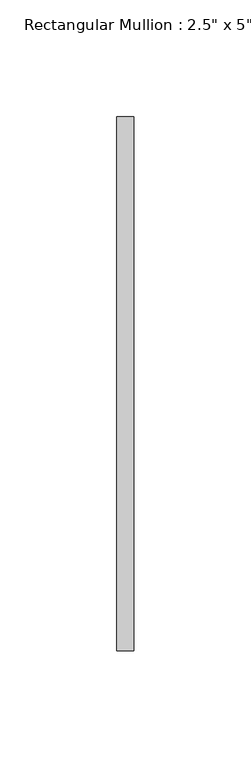
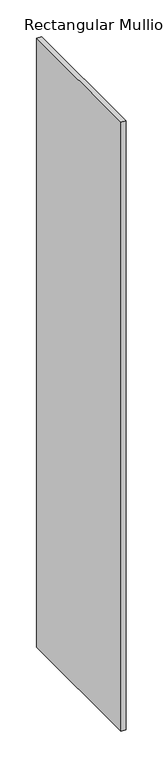
"""IFC4 building model written with IfcOpenShell, lengths in millimetres: member geometry."""

from ifc_helpers import new_model, si_unit, frame, origin, place, context, project, spatial, polyline, outline, extrude, source, transform, mapped, element, save


def member_9004b0e6(model_context):
    return source(origin(), model_context, "Body", "SweptSolid", [
        extrude(outline(polyline([(0.0, 114.3), (0.0, -114.3), (-7.239, -114.3), (-7.239, 114.3), (0.0, 114.3)])), frame((0.0, 0.0, -1005.1415), z_axis=(0.0, 0.0, 1.0), x_axis=(1.0, 0.0, 0.0)), (0.0, 0.0, 1.0), 1005.1415),
    ])


if __name__ == "__main__":
    model = new_model("IFC4")
    model_context = context("Model", 3, world=origin())
    ifc_project = project(units=[si_unit("LENGTHUNIT", "METRE", prefix="MILLI")], contexts=[model_context])
    site = spatial("IfcSite", under=ifc_project)
    building = spatial("IfcBuilding", under=site)
    placement = place(None, origin())
    member_shape = member_9004b0e6(model_context)
    element("IfcMember", 1, ObjectType="Rectangular Mullion : 2.5\" x 5\" rectangular", at=placement, inside=building, context=model_context, shape_type="MappedRepresentation", body=[
        mapped(member_shape, transform((0.0, 0.0, 0.0), x_axis=(1.0, 0.0, 0.0), y_axis=(0.0, 1.0, 0.0), z_axis=(0.0, 0.0, 1.0))),
    ])
    save(model, "model.ifc")

# Revit data of these elements
# Type "Rectangular Mullion : 2.5\" x 5\" rectangular"
#   built-in parameter 1007304 = 0.75 (stored number, unit not read)
#   built-in parameter 1007301 = 0.011875 (stored number, unit not read)
#   built-in parameter 1007300 = 0.011875 (stored number, unit not read)
# Element 1 (IfcMember, "Rectangular Mullion : 2.5\" x 5\" rectangular")
#   Materials on its faces: "WINDOW GLASS MATERIAL"
# Materials
#   "WINDOW GLASS MATERIAL": class "Generic", colour RGB 120 120 120, transparency 0, Cost = 0
